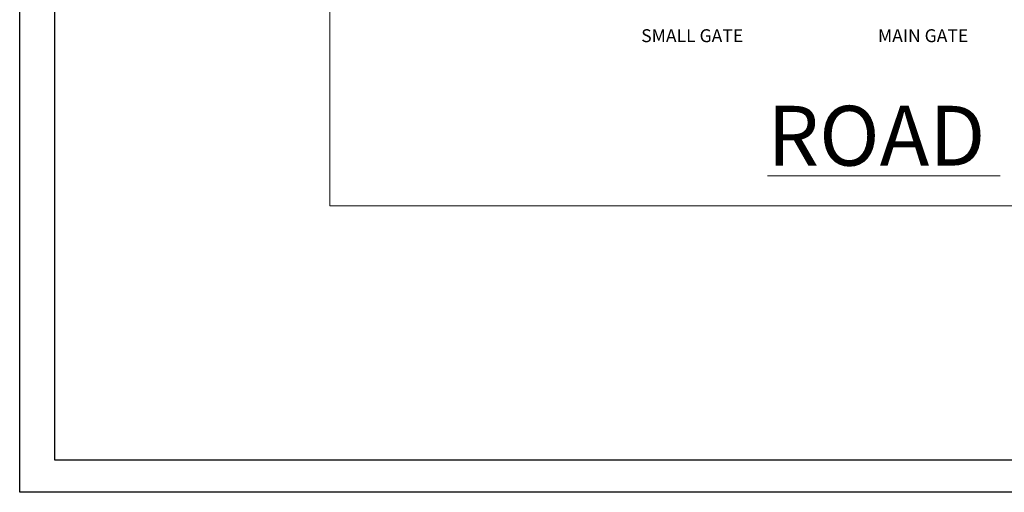
# Model space of a CAD drawing. Units: inches. Extents: x 0 to 4258, y 0 to 3769.
# Tile 1 of 30: x 3476 to 3859, y 2750 to 2933. Entities that reach past the tile are written whole.
import ezdxf

# ---------------------------------------------------------------- set-up
doc = ezdxf.new("R2010")
doc.units = ezdxf.units.IN
doc.header["$MEASUREMENT"] = 0
for name, color, linetype, lineweight in [('A-ANNO-TEXT', 250, 'Continuous', 18), ('A-ANNO-TTLB', 250, 'Continuous', 25), ('C-ROAD', 250, 'Continuous', 18)]:
    doc.layers.add(name, color=color, linetype=linetype, lineweight=lineweight)
doc.styles.get("Standard").update_dxf_attribs({"font": 'arial.ttf'})

msp = doc.modelspace()

# ---------------------------------------------------------------- linework, layer by layer
at = {"layer": 'A-ANNO-TEXT'}
msp.add_line((3766.749, 2872.626), (3857.287, 2872.626), dxfattribs=at)
at = {"layer": 'A-ANNO-TTLB'}
for p, q in [((3476.156, 2762.335), (3476.156, 3768.679)), ((3489.722, 3758.41), (3489.722, 2762.335)), ((3476.156, 2749.714), (3476.156, 2762.335)), ((3489.722, 2762.335), (4244.279, 2762.335)), ((4257.673, 2749.714), (3476.156, 2749.714))]:
    msp.add_line(p, q, dxfattribs=at)
at = {"layer": 'C-ROAD'}
for p, q in [((3596.728, 2936.793), (3596.728, 2860.957)), ((3596.728, 2860.957), (4133.199, 2860.957))]:
    msp.add_line(p, q, dxfattribs=at)

# ---------------------------------------------------------------- texts
at = {"layer": 'A-ANNO-TEXT'}
for s, height, p in [('SMALL GATE', 5, (3717.713, 2924.476)), ('MAIN GATE', 5, (3809.734, 2924.476)), ('ROAD', 23.2379, (3766.749, 2876.51))]:
    msp.add_text(s, height=height, dxfattribs=at).set_placement(p)

doc.saveas('drawing.dxf')
